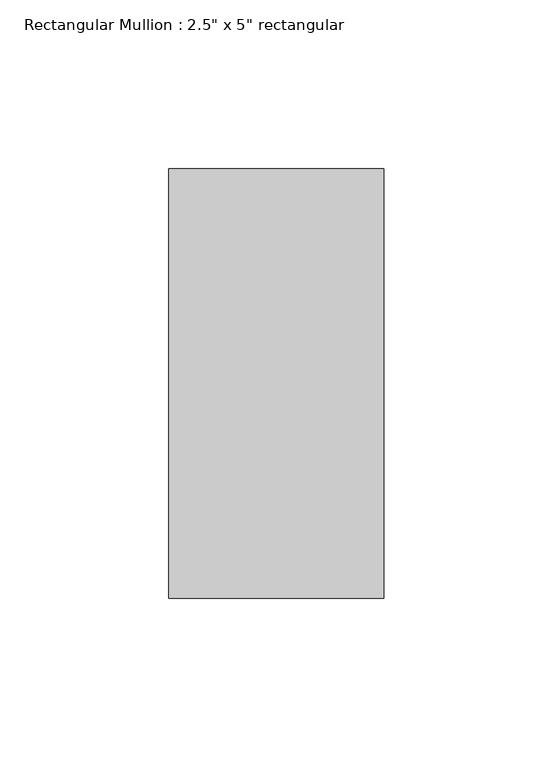
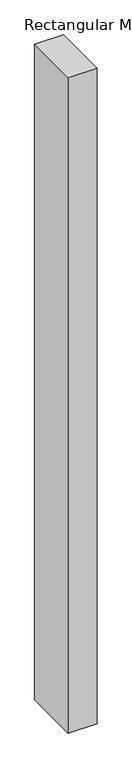
"""IFC4 building model written with IfcOpenShell, lengths in millimetres: member geometry."""

from ifc_helpers import new_model, si_unit, frame, origin, place, context, project, spatial, polyline, outline, extrude, source, transform, mapped, element, save


def member_e5016be8(model_context):
    return source(origin(), model_context, "Body", "SweptSolid", [
        extrude(outline(polyline([(0.0, 63.5), (0.0, -63.5), (-63.5, -63.5), (-63.5, 63.5), (0.0, 63.5)])), frame((0.0, 0.0, -1523.1033231), z_axis=(0.0, 0.0, 1.0), x_axis=(1.0, 0.0, 0.0)), (0.0, 0.0, 1.0), 1523.1033231),
    ])


if __name__ == "__main__":
    model = new_model("IFC4")
    model_context = context("Model", 3, world=origin())
    ifc_project = project(units=[si_unit("LENGTHUNIT", "METRE", prefix="MILLI")], contexts=[model_context])
    site = spatial("IfcSite", under=ifc_project)
    building = spatial("IfcBuilding", under=site)
    placement = place(None, origin())
    member_shape = member_e5016be8(model_context)
    element("IfcMember", 1, ObjectType="Rectangular Mullion : 2.5\" x 5\" rectangular", at=placement, inside=building, context=model_context, shape_type="MappedRepresentation", body=[
        mapped(member_shape, transform((0.0, 0.0, 0.0), x_axis=(1.0, 0.0, 0.0), y_axis=(0.0, 1.0, 0.0), z_axis=(0.0, 0.0, 1.0))),
    ])
    save(model, "model.ifc")

# Revit data of these elements
# Type "Rectangular Mullion : 2.5\" x 5\" rectangular"
#   built-in parameter 1007304 = 0.416667 (stored number, unit not read)
#   built-in parameter 1007301 = 0.104167 (stored number, unit not read)
#   built-in parameter 1007300 = 0.104167 (stored number, unit not read)
# Element 1 (IfcMember, "Rectangular Mullion : 2.5\" x 5\" rectangular")
#   Materials on its faces: "Aluminum"
# Materials
#   "Aluminum": class "Metal", colour RGB 247 247 247, transparency 0, Description = "Aluminum 6061", Cost = 0
